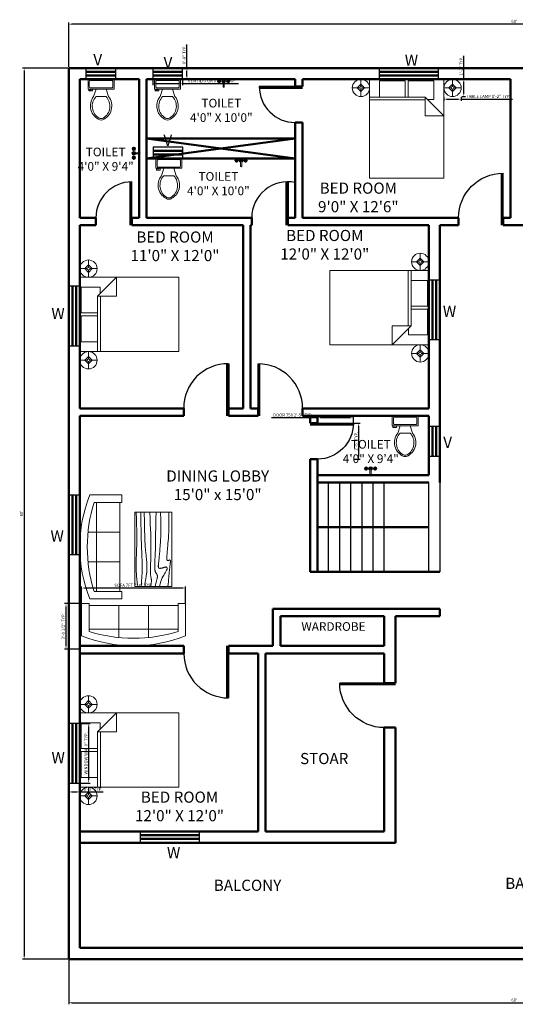
# Model space of a CAD drawing. Units: inches. Extents: x 2663 to 4539, y 2314 to 3111.
# Tile 3 of 4: x 3742 to 4143, y 2316 to 3111. Entities that reach past the tile are written whole.
import ezdxf

# ---------------------------------------------------------------- set-up
doc = ezdxf.new("R2010")
doc.units = ezdxf.units.IN
for name, color, linetype, lineweight in [('A-ANNO-DIMS', 2, 'Continuous', 18), ('A-ANNO-TEXT', 7, 'Continuous', 18), ('A-AREA-IDEN', 3, 'Continuous', 25), ('A-DOOR', 4, 'Continuous', 25), ('A-FLOR-FIXT', 8, 'Continuous', 18), ('A-FLOR-STRS', 2, 'Continuous', 25), ('A-FURN', 8, 'Continuous', 18), ('A-GLAZ', 3, 'Continuous', 25), ('A-WALL', 7, 'Continuous', 50)]:
    doc.layers.add(name, color=color, linetype=linetype, lineweight=lineweight)
doc.styles.get("Standard").update_dxf_attribs({"font": 'arial.ttf'})
doc.dimstyles.new('ISO-25', dxfattribs={"dimtxt": 2.5, "dimasz": 2.5, "dimexe": 1.25, "dimexo": 0.625, "dimtad": 1, "dimdec": 0, "dimlunit": 3, "dimtxsty": 'Standard', "dimcen": 2.5, "dimadec": 0, "dimazin": 0, "dimtfac": 1, "dimtdec": 0, "dimtmove": 0, "dimatfit": 3, "dimfxl": 1, "dimarcsym": 0})

# ---------------------------------------------------------------- blocks, each defined once
blk = doc.blocks.new('Toilet - top')
for p, q in [((9.5, -6), (9.5, -2)), ((-10, -8.5), (-8, -8.5)), ((-10, -9.5), (-10, -8.5)), ((-7, -9.5), (-10, -9.5)), ((-8, -8.5), (-8, -8)), ((-7, -8), (-7, -9.5)), ((-4, -8), (-6, -14)), ((4, -14), (-4, -14)), ((4, -8), (6, -14))]:
    blk.add_line(p, q)
blk.add_lwpolyline([(10.5, -8), (10.5, 0), (-10.5, 0), (-10.5, -8)], close=True)
for points in [[(-9.5, -2), (-9.5, -6)], [(8.5, -1), (-8.5, -1)], [(-8.5, -7), (8.5, -7)]]:
    blk.add_lwpolyline(points)
for centre, radius, start, end in [((-8.62, -1.88), 0.884, 81.8699, 188.1301), ((-8.62, -6.12), 0.884, 171.8699, 278.1301), ((8.62, -1.88), 0.884, 351.8699, 98.1301), ((8.62, -6.12), 0.884, 261.8699, 8.1301), ((3.52, -21.58), 12.17, 141.46911, 247.97143), ((4.2, -21.82), 11.33, 136.36773, 238.94682), ((-3.52, -21.58), 12.17, 292.02843, 38.53071), ((-4.2, -21.82), 11.33, 301.05301, 43.63209), ((0, -27.88), 4, 245.73182, 294.26817), ((0, -29), 4, 254.86053, 285.13947)]:
    blk.add_arc(centre, radius, start, end)
blk = doc.blocks.new('Faucet - Bathroom top')
for p, q in [((-4.107, 0.125), (-4.375, 0.125)), ((-3.75, 0.4788), (-3.75, 0.75)), ((-3.5, 0.482), (-3.5, 0.75)), ((-3.1461, 0.125), (-2.875, 0.125)), ((3.143, 0.125), (2.875, 0.125)), ((3.5, 0.4788), (3.5, 0.75)), ((3.75, 0.482), (3.75, 0.75)), ((4.1039, 0.125), (4.375, 0.125)), ((-4.1039, -0.125), (-4.375, -0.125)), ((-3.75, -0.4821), (-3.75, -0.75)), ((-3.5, -0.4789), (-3.5, -0.75)), ((-3.143, -0.125), (-2.875, -0.125)), ((-0.5, -0.8639), (-0.5, -4.5)), ((0.5, -4.5), (0.5, -0.8631)), ((3.1461, -0.125), (2.875, -0.125)), ((3.5, -0.4821), (3.5, -0.75)), ((3.75, -0.4789), (3.75, -0.75)), ((4.107, -0.125), (4.375, -0.125))]:
    blk.add_line(p, q)
for centre, radius in [((-3.625, 0), 1.375), ((-4.625, 0), 0.2795), ((-3.625, 0), 0.5), ((-3.625, 1), 0.2795), ((-2.625, 0), 0.2795), ((0, 0), 0.5), ((3.625, 0), 1.375), ((2.625, 0), 0.2795), ((3.625, 0), 0.5), ((3.625, 1), 0.2795), ((4.625, 0), 0.2795), ((-3.625, -1), 0.2795), ((3.625, -1), 0.2795)]:
    blk.add_circle(centre, radius)
for centre, radius, start, end in [((-3.625, 0), 1, 105.2407, 164.2093), ((-3.625, 0), 1, 16.44125, 74.07887), ((0, 0), 1.5, 289.6514, 250.3603), ((0, 0), 1, 300.3431, 239.7554), ((3.625, 0), 1, 106.12, 164.0884), ((3.625, 0), 1, 16.23422, 73.90469), ((-3.625, 0), 1, 196.2342, 253.9047), ((-3.625, 0), 1, 286.12, 344.0884), ((0, -4.5), 0.5, 180, 0), ((3.625, 0), 1, 196.4413, 254.0789), ((3.625, 0), 1, 285.2407, 344.2093)]:
    blk.add_arc(centre, radius, start, end)
blk = doc.blocks.new('Bed - Queen')
for p, q in [((0, -80.00003), (0, 0)), ((0, 0), (59.99999, 0)), ((59.99999, 0), (59.99999, -80.00003)), ((7.99999, -1.2), (28.79998, -1.2)), ((7.99999, -14.4), (7.99999, -1.2)), ((28.79998, -1.2), (28.79998, -14.4)), ((31.19999, -1.2), (51.99999, -1.2)), ((31.19999, -14.4), (31.19999, -1.2)), ((51.99999, -1.2), (51.99999, -16.4)), ((0, -14.4), (44.8, -14.4)), ((59.99999, -29.6), (44.8, -14.4)), ((44.8, -14.4), (44.8, -29.6)), ((44.8, -16.8), (0, -16.8)), ((51.99999, -16.4), (46.79936, -16.4)), ((44.8, -29.6), (59.99999, -29.6)), ((59.99999, -80.00003), (0, -80.00003))]:
    blk.add_line(p, q)
blk = doc.blocks.new('Lamp - Table')
for p, q in [((-1, 0), (-7, 0)), ((0, 3), (-3, 0)), ((-3, 0), (0, -3)), ((0, 7), (0, 1)), ((3, 0), (0, 3)), ((0, -3), (3, 0)), ((1, 0), (7, 0)), ((0, -1), (0, -7))]:
    blk.add_line(p, q)
for radius in [7, 1]:
    blk.add_circle((0, 0), radius)
blk = doc.blocks.new('Sofa - Roundback 7 ft.')
for p, q in [((-12.00002, -32.4421), (-12.00003, -6.5971)), ((11.99997, -32.4421), (11.99998, -6.5971)), ((-36.000027, -34), (-36.000027, -11.4696)), ((-35.999844, -13.3819), (35.9998, -13.3819)), ((35.99998, -34), (35.99998, -11.4696)), ((-36.000027, -32.4421), (35.99998, -32.4421))]:
    blk.add_line(p, q)
for points in [[(-36.000027, -34), (-42.000027, -34), (-42.000027, -8)], [(41.99998, -8), (41.99998, -34), (35.99998, -34)]]:
    blk.add_lwpolyline(points)
for centre, radius, start, end in [((0, -114.25), 114.25, 68.43141, 111.5686), ((-0.00001, -127.1968), 121.1968, 72.72033, 107.2797)]:
    blk.add_arc(centre, radius, start, end)
blk = doc.blocks.new('Table - Rectangular Woodgrain 60 x 30 in.')
for p, q in [((0, 0), (0, -30)), ((60, 0), (0, 0)), ((60, -30), (60, 0)), ((0, -30), (60, -30))]:
    blk.add_line(p, q)
for points in [[(0, -2.4), (4.8155, -2.418), (9.0302, -2.4688), (12.709, -2.5477), (15.9167, -2.65), (18.7181, -2.7711), (21.1781, -2.9063), (23.3616, -3.0508), (25.3333, -3.2), (27.1477, -3.3495), (28.8172, -3.4958), (30.3437, -3.636), (31.7291, -3.7667), (32.9756, -3.8849), (34.0849, -3.9875), (35.059, -4.0714), (35.9, -4.1334), (36.6114, -4.1711), (37.2041, -4.1854), (37.6906, -4.1779), (38.0833, -4.15), (38.3948, -4.1034), (38.6375, -4.0396), (38.8239, -3.9602), (38.9666, -3.8667), (39.0764, -3.7608), (39.1573, -3.6448), (39.2116, -3.521), (39.2416, -3.3917), (39.2498, -3.2593), (39.2385, -3.1261), (39.21, -2.9944), (39.1666, -2.8667), (39.111, -2.7447), (39.0468, -2.6281), (38.978, -2.5163), (38.9083, -2.4083), (38.8418, -2.3035), (38.7823, -2.201), (38.7337, -2.1001), (38.7, -2), (38.6844, -1.9003), (38.6875, -1.8021), (38.7094, -1.707), (38.75, -1.6167), (38.8094, -1.5326), (38.8875, -1.4563), (38.9844, -1.3893), (39.1, -1.3333), (39.2351, -1.2896), (39.3937, -1.2583), (39.5804, -1.2396), (39.8, -1.2333), (40.057, -1.2396), (40.3562, -1.2583), (40.7023, -1.2896), (41.1, -1.3333), (41.5547, -1.3895), (42.0755, -1.4573), (42.6721, -1.5361), (43.3542, -1.625), (44.1316, -1.7233), (45.014, -1.8302), (46.0114, -1.9449), (47.1333, -2.0667), (48.3862, -2.1947), (49.7625, -2.3281), (51.2513, -2.4663), (52.8416, -2.6083), (54.5226, -2.7535), (56.2833, -2.9011), (58.1127, -3.0501), (60, -3.2)], [(0, -9.2), (6.5759, -9.0858), (11.9385, -9.0365), (16.2527, -9.0418), (19.6833, -9.0917), (22.3952, -9.1759), (24.5531, -9.2844), (26.322, -9.4069), (27.8666, -9.5333), (29.3241, -9.6553), (30.7203, -9.7719), (32.0532, -9.8837), (33.3208, -9.9917), (34.5213, -10.0965), (35.6526, -10.199), (36.7128, -10.2999), (37.7, -10.4), (38.6129, -10.4996), (39.4531, -10.5969), (40.223, -10.6895), (40.925, -10.775), (41.5613, -10.8512), (42.1344, -10.9156), (42.6465, -10.966), (43.1, -11), (43.4976, -11.0158), (43.8437, -11.0136), (44.143, -10.9942), (44.4, -10.9583), (44.6195, -10.9069), (44.8062, -10.8406), (44.9648, -10.7603), (45.1, -10.6667), (45.2155, -10.5598), (45.3114, -10.4365), (45.3871, -10.2929), (45.4416, -10.125), (45.4743, -9.929), (45.4844, -9.7011), (45.4709, -9.4371), (45.4333, -9.1333), (45.3716, -8.7883), (45.2896, -8.4104), (45.1919, -8.0107), (45.0833, -7.6), (44.9685, -7.1893), (44.8521, -6.7896), (44.7388, -6.4117), (44.6333, -6.0667), (44.54, -5.7628), (44.4614, -5.4979), (44.4001, -5.2675), (44.3583, -5.0667), (44.3384, -4.8909), (44.3427, -4.7354), (44.3736, -4.5956), (44.4333, -4.4667), (44.5236, -4.3453), (44.6427, -4.2333), (44.7884, -4.1339), (44.9583, -4.05), (45.1501, -3.9849), (45.3614, -3.9417), (45.59, -3.9234), (45.8333, -3.9333), (46.0915, -3.9749), (46.3734, -4.0531), (46.6906, -4.1736), (47.0542, -4.3417), (47.4756, -4.5629), (47.9661, -4.8427), (48.5372, -5.1866), (49.2, -5.6), (49.9676, -6.0844), (50.8594, -6.625), (51.8965, -7.2031), (53.1, -7.8), (54.491, -8.3969), (56.0906, -8.975), (57.9199, -9.5156), (60, -10)], [(0, -12.8), (5.1847, -12.9322), (9.6213, -13.0323), (13.3963, -13.1059), (16.5958, -13.1583), (19.3063, -13.1952), (21.614, -13.2219), (23.6054, -13.2439), (25.3666, -13.2667), (26.9728, -13.2947), (28.4531, -13.3281), (29.8256, -13.3663), (31.1083, -13.4083), (32.3191, -13.4535), (33.476, -13.501), (34.597, -13.5501), (35.7, -13.6), (36.7984, -13.6497), (37.8875, -13.6979), (38.9578, -13.743), (40, -13.7833), (41.0047, -13.8174), (41.9625, -13.8438), (42.864, -13.8607), (43.7, -13.8667), (44.4631, -13.8604), (45.1552, -13.8417), (45.7801, -13.8104), (46.3416, -13.7667), (46.8439, -13.7104), (47.2906, -13.6417), (47.6858, -13.5604), (48.0333, -13.4667), (48.3375, -13.3608), (48.6042, -13.2448), (48.8396, -13.121), (49.05, -12.9917), (49.2417, -12.8593), (49.4208, -12.7261), (49.5937, -12.5944), (49.7667, -12.4667), (49.9452, -12.3451), (50.1323, -12.2313), (50.3303, -12.1268), (50.5416, -12.0333), (50.7686, -11.9524), (51.0135, -11.8854), (51.2788, -11.8341), (51.5666, -11.8), (51.8785, -11.7843), (52.2116, -11.7865), (52.562, -11.8059), (52.926, -11.8417), (53.2998, -11.8931), (53.6795, -11.9594), (54.0614, -12.0397), (54.4416, -12.1333), (54.8223, -12.2401), (55.2293, -12.3625), (55.6942, -12.5037), (56.2489, -12.6667), (56.9251, -12.8547), (57.7545, -13.0708), (58.7689, -13.3182), (60, -13.6)], [(0, -18), (5.124, -17.7273), (9.6609, -17.5057), (13.6705, -17.3303), (17.2125, -17.1958), (20.3467, -17.0973), (23.1328, -17.0297), (25.6307, -16.9878), (27.9, -16.9667), (29.9928, -16.9617), (31.9302, -16.9703), (33.7254, -16.9907), (35.3917, -17.0208), (36.9423, -17.0588), (38.3906, -17.1026), (39.7499, -17.1503), (41.0333, -17.2), (42.2519, -17.2496), (43.4073, -17.2969), (44.4986, -17.3395), (45.525, -17.375), (46.4858, -17.4012), (47.3802, -17.4156), (48.2074, -17.416), (48.9667, -17.4), (49.6583, -17.3662), (50.2872, -17.3167), (50.8595, -17.2547), (51.3812, -17.1833), (51.8584, -17.1057), (52.2971, -17.025), (52.7034, -16.9443), (53.0833, -16.8667), (53.443, -16.7951), (53.789, -16.7313), (54.128, -16.6768), (54.4666, -16.6334), (54.8115, -16.6024), (55.1693, -16.5854), (55.5465, -16.5841), (55.95, -16.6), (56.3828, -16.6337), (56.8346, -16.6823), (57.2915, -16.7418), (57.7396, -16.8084), (58.165, -16.878), (58.5539, -16.9469), (58.8924, -17.0111), (59.1666, -17.0667), (59.3679, -17.1107), (59.5078, -17.1438), (59.6032, -17.1675), (59.6708, -17.1833), (59.7275, -17.193), (59.7901, -17.1979), (59.8753, -17.1998), (60, -17.2)], [(0, -22.4), (8.0098, -22.2501), (14.4094, -22.1011), (19.4168, -21.9535), (23.25, -21.8083), (26.1269, -21.6663), (28.2656, -21.5281), (29.884, -21.3947), (31.2, -21.2667), (32.3967, -21.1448), (33.5172, -21.0292), (34.5697, -20.9198), (35.5625, -20.8167), (36.5037, -20.7198), (37.4015, -20.6292), (38.2642, -20.5448), (39.1, -20.4667), (39.9164, -20.3951), (40.7187, -20.3313), (41.5117, -20.2768), (42.3, -20.2333), (43.0883, -20.2024), (43.8812, -20.1854), (44.6836, -20.1841), (45.5, -20.2), (46.3328, -20.234), (47.1747, -20.2844), (48.0163, -20.3488), (48.8479, -20.425), (49.66, -20.5106), (50.4429, -20.6031), (51.1872, -20.7004), (51.8833, -20.8), (52.5246, -20.8999), (53.1166, -20.9995), (53.6681, -21.0983), (54.1875, -21.1958), (54.6834, -21.2919), (55.1646, -21.3859), (55.6394, -21.4777), (56.1167, -21.5667), (56.6028, -21.6515), (57.0961, -21.7266), (57.5929, -21.7852), (58.0896, -21.8208), (58.5823, -21.8268), (59.0674, -21.7964), (59.5412, -21.723), (60, -21.6)], [(0, -25.2), (8.6355, -25.0504), (15.7026, -24.9031), (21.4049, -24.7606), (25.9458, -24.625), (29.529, -24.4988), (32.3578, -24.3844), (34.6359, -24.284), (36.5667, -24.2), (38.3213, -24.1341), (39.9417, -24.0854), (41.437, -24.0523), (42.8167, -24.0333), (44.0901, -24.0268), (45.2667, -24.0313), (46.3557, -24.0451), (47.3667, -24.0667), (48.309, -24.0947), (49.1928, -24.1287), (50.0284, -24.168), (50.826, -24.2125), (51.5959, -24.2617), (52.3483, -24.3151), (53.0935, -24.3725), (53.8417, -24.4334), (54.6009, -24.497), (55.3699, -24.561), (56.1454, -24.6226), (56.9239, -24.6792), (57.7021, -24.7279), (58.4764, -24.7662), (59.2435, -24.7911), (60, -24.8)], [(0, -28.8), (5.6867, -28.6681), (10.45, -28.5698), (14.407, -28.5012), (17.675, -28.4584), (20.3711, -28.4374), (22.6125, -28.4344), (24.5164, -28.4455), (26.2, -28.4667), (27.762, -28.4947), (29.2276, -28.5281), (30.6033, -28.5663), (31.8958, -28.6084), (33.1118, -28.6535), (34.2578, -28.7011), (35.3405, -28.7501), (36.3666, -28.8), (37.3443, -28.8497), (38.288, -28.8974), (39.2137, -28.9412), (40.1375, -28.9792), (41.0753, -29.0093), (42.0432, -29.0297), (43.0572, -29.0384), (44.1333, -29.0333), (45.2936, -29.0114), (46.5843, -28.9641), (48.0579, -28.8816), (49.7666, -28.7542), (51.7629, -28.5721), (54.0989, -28.3255), (56.8272, -28.0048), (60, -27.6)]]:
    blk.add_lwpolyline(points)
blk = doc.blocks.new('*D14')
at = {"layer": 'A-ANNO-DIMS', "color": 0, "lineweight": -2, "transparency": 16777216}
for p, q in [((3781.84, 3072.75), (3781.84, 3108.85)), ((4499.34, 3107.6), (3784.34, 3107.6)), ((4501.84, 3072.75), (4501.84, 3108.85))]:
    blk.add_line(p, q, dxfattribs=at)
at = {"layer": 'A-ANNO-DIMS', "color": 0, "transparency": 16777216}
for points in [[(3784.34, 3108.02), (3784.34, 3107.19), (3781.84, 3107.6)], [(4499.34, 3108.02), (4499.34, 3107.19), (4501.84, 3107.6)]]:
    blk.add_solid(points, dxfattribs=at)
at = {"layer": 'Defpoints', "color": 0, "transparency": 16777216}
for p in [(3781.84, 3107.6), (3781.84, 3072.12), (4501.84, 3072.12)]:
    blk.add_point(p, dxfattribs=at)
at = {"layer": 'A-ANNO-DIMS', "color": 0, "transparency": 16777216, "insert": (4141.84, 3109.51), "char_height": 2.5, "attachment_point": 5}
blk.add_mtext("60'", dxfattribs=at)
blk = doc.blocks.new('*D16')
at = {"layer": 'A-ANNO-DIMS', "color": 0, "lineweight": -2, "transparency": 16777216}
for p, q in [((3781.21, 3072.12), (3744.61, 3072.12)), ((3745.86, 3069.62), (3745.86, 2354.62)), ((3781.21, 2352.12), (3744.61, 2352.12))]:
    blk.add_line(p, q, dxfattribs=at)
at = {"layer": 'A-ANNO-DIMS', "color": 0, "transparency": 16777216}
for points in [[(3745.45, 3069.62), (3746.28, 3069.62), (3745.86, 3072.12)], [(3745.45, 2354.62), (3746.28, 2354.62), (3745.86, 2352.12)]]:
    blk.add_solid(points, dxfattribs=at)
at = {"layer": 'Defpoints', "color": 0, "transparency": 16777216}
for p in [(3781.84, 3072.12), (3745.86, 2352.12), (3781.84, 2352.12)]:
    blk.add_point(p, dxfattribs=at)
at = {"layer": 'A-ANNO-DIMS', "color": 0, "transparency": 16777216, "insert": (3743.96, 2712.12), "char_height": 2.5, "attachment_point": 5, "rotation": 90}
blk.add_mtext("60'", dxfattribs=at)
blk = doc.blocks.new('*D17')
at = {"layer": 'A-ANNO-DIMS', "color": 0, "lineweight": -2, "transparency": 16777216}
for p, q in [((3781.84, 2352.78), (3781.84, 2315.51)), ((4501.84, 2351.5), (4501.84, 2315.51)), ((3784.34, 2316.76), (4499.34, 2316.76))]:
    blk.add_line(p, q, dxfattribs=at)
at = {"layer": 'A-ANNO-DIMS', "color": 0, "transparency": 16777216}
for points in [[(3784.34, 2317.18), (3784.34, 2316.35), (3781.84, 2316.76)], [(4499.34, 2317.18), (4499.34, 2316.35), (4501.84, 2316.76)]]:
    blk.add_solid(points, dxfattribs=at)
at = {"layer": 'Defpoints', "color": 0, "transparency": 16777216}
for p in [(3781.84, 2353.4), (4501.84, 2352.12), (4501.84, 2316.76)]:
    blk.add_point(p, dxfattribs=at)
at = {"layer": 'A-ANNO-DIMS', "color": 0, "transparency": 16777216, "insert": (4141.84, 2318.67), "char_height": 2.5, "attachment_point": 5}
blk.add_mtext("60'", dxfattribs=at)
blk = doc.blocks.new('WIN-1200')
for p, q in [((0, 48), (0, 0)), ((9, 48), (0, 48)), ((0, 48), (0, 48)), ((9, 0), (9, 48)), ((0, 0), (9, 0))]:
    blk.add_line(p, q)
blk = doc.blocks.new('VENT-600')
for p, q in [((24, 9), (0, 9)), ((0, 9), (0, 0)), ((24, 0), (24, 9)), ((0, 0), (24, 0))]:
    blk.add_line(p, q)
blk = doc.blocks.new('DOOR-750')
blk.add_line((2901.63, 3055.91), (2872.63, 3055.91))
blk.add_arc((2901.63, 3055.91), 29, 180, 270)
blk = doc.blocks.new('DOOR-900')
blk.add_line((3071.63, 2949.91), (3071.63, 2985.91))
blk.add_arc((3071.63, 2949.91), 36, 0, 90)
blk = doc.blocks.new('*D24')
at = {"layer": 'A-ANNO-DIMS', "color": 0, "lineweight": -2, "transparency": 16777216}
for p, q in [((4084.96, 3048.5), (4084.96, 3045.77)), ((4098.96, 3048.5), (4098.96, 3045.77)), ((4087.46, 3047.02), (4096.46, 3047.02)), ((4098.96, 3047.02), (4140.53, 3047.02))]:
    blk.add_line(p, q, dxfattribs=at)
at = {"layer": 'A-ANNO-DIMS', "color": 0, "transparency": 16777216}
for points in [[(4087.46, 3047.44), (4087.46, 3046.61), (4084.96, 3047.02)], [(4096.46, 3047.44), (4096.46, 3046.61), (4098.96, 3047.02)]]:
    blk.add_solid(points, dxfattribs=at)
at = {"layer": 'Defpoints', "color": 0, "transparency": 16777216}
for p in [(4084.96, 3049.12), (4098.96, 3049.12), (4098.96, 3047.02)]:
    blk.add_point(p, dxfattribs=at)
at = {"layer": 'A-ANNO-DIMS', "color": 0, "transparency": 16777216, "insert": (4120.99, 3048.91), "char_height": 2.5, "attachment_point": 5}
blk.add_mtext('TABLE LAMP 1\'-2" TYP.', dxfattribs=at)
blk = doc.blocks.new('*D25')
at = {"layer": 'A-ANNO-DIMS', "color": 0, "lineweight": -2, "transparency": 16777216}
for p, q in [((4101.06, 3063.12), (4101.06, 3081.88)), ((4099.58, 3063.12), (4102.31, 3063.12)), ((4101.06, 3051.62), (4101.06, 3060.62)), ((4099.58, 3049.12), (4102.31, 3049.12))]:
    blk.add_line(p, q, dxfattribs=at)
at = {"layer": 'A-ANNO-DIMS', "color": 0, "transparency": 16777216}
for points in [[(4100.64, 3060.62), (4101.48, 3060.62), (4101.06, 3063.12)], [(4100.64, 3051.62), (4101.48, 3051.62), (4101.06, 3049.12)]]:
    blk.add_solid(points, dxfattribs=at)
at = {"layer": 'Defpoints', "color": 0, "transparency": 16777216}
for p in [(4098.96, 3063.12), (4101.06, 3063.12), (4098.96, 3049.12)]:
    blk.add_point(p, dxfattribs=at)
at = {"layer": 'A-ANNO-DIMS', "color": 0, "transparency": 16777216, "insert": (4099.18, 3073.75), "char_height": 2.5, "attachment_point": 5, "rotation": 90}
blk.add_mtext('1\'-2" TYP.', dxfattribs=at)
blk = doc.blocks.new('*D26')
at = {"layer": 'A-ANNO-DIMS', "color": 0, "lineweight": -2, "transparency": 16777216}
for p, q in [((3791.46, 2542.34), (3799.29, 2542.34)), ((3798.04, 2496.84), (3798.04, 2539.84)), ((3791.46, 2494.34), (3799.29, 2494.34))]:
    blk.add_line(p, q, dxfattribs=at)
at = {"layer": 'A-ANNO-DIMS', "color": 0, "transparency": 16777216}
for points in [[(3797.62, 2539.84), (3798.46, 2539.84), (3798.04, 2542.34)], [(3797.62, 2496.84), (3798.46, 2496.84), (3798.04, 2494.34)]]:
    blk.add_solid(points, dxfattribs=at)
at = {"layer": 'Defpoints', "color": 0, "transparency": 16777216}
for p in [(3790.84, 2542.34), (3798.04, 2542.34), (3790.84, 2494.34)]:
    blk.add_point(p, dxfattribs=at)
at = {"layer": 'A-ANNO-DIMS', "color": 0, "transparency": 16777216, "insert": (3796.12, 2518.34), "char_height": 2.5, "attachment_point": 5, "rotation": 90}
blk.add_mtext('WINDOW W 4\'-0" TYP.', dxfattribs=at)
blk = doc.blocks.new('*D27')
at = {"layer": 'A-ANNO-DIMS', "color": 0, "lineweight": -2, "transparency": 16777216}
for p, q in [((3781.84, 2493.72), (3781.84, 2485.89)), ((3790.84, 2493.72), (3790.84, 2485.89)), ((3784.34, 2487.14), (3788.34, 2487.14)), ((3790.84, 2487.14), (3809.83, 2487.14))]:
    blk.add_line(p, q, dxfattribs=at)
at = {"layer": 'A-ANNO-DIMS', "color": 0, "transparency": 16777216}
for points in [[(3784.34, 2487.56), (3784.34, 2486.73), (3781.84, 2487.14)], [(3788.34, 2487.56), (3788.34, 2486.73), (3790.84, 2487.14)]]:
    blk.add_solid(points, dxfattribs=at)
at = {"layer": 'Defpoints', "color": 0, "transparency": 16777216}
for p in [(3781.84, 2494.34), (3790.84, 2494.34), (3790.84, 2487.14)]:
    blk.add_point(p, dxfattribs=at)
at = {"layer": 'A-ANNO-DIMS', "color": 0, "transparency": 16777216, "insert": (3801.58, 2489.05), "char_height": 2.5, "attachment_point": 5}
blk.add_mtext('0\'-9" TYP.', dxfattribs=at)
blk = doc.blocks.new('*D30')
at = {"layer": 'A-ANNO-DIMS', "color": 0, "lineweight": -2, "transparency": 16777216}
for p, q in [((3849.76, 3062.5), (3849.76, 3058.27)), ((3852.26, 3059.52), (3871.26, 3059.52)), ((3873.76, 3062.5), (3873.76, 3058.27)), ((3873.76, 3059.52), (3919.08, 3059.52))]:
    blk.add_line(p, q, dxfattribs=at)
at = {"layer": 'A-ANNO-DIMS', "color": 0, "transparency": 16777216}
for points in [[(3852.26, 3059.94), (3852.26, 3059.11), (3849.76, 3059.52)], [(3871.26, 3059.94), (3871.26, 3059.11), (3873.76, 3059.52)]]:
    blk.add_solid(points, dxfattribs=at)
at = {"layer": 'Defpoints', "color": 0, "transparency": 16777216}
for p in [(3849.76, 3063.12), (3873.76, 3063.12), (3873.76, 3059.52)]:
    blk.add_point(p, dxfattribs=at)
at = {"layer": 'A-ANNO-DIMS', "color": 0, "transparency": 16777216, "insert": (3897.67, 3061.44), "char_height": 2.5, "attachment_point": 5}
blk.add_mtext('VENTILATOR V 2\'-0" TYP.', dxfattribs=at)
blk = doc.blocks.new('*D31')
at = {"layer": 'A-ANNO-DIMS', "color": 0, "lineweight": -2, "transparency": 16777216}
for p, q in [((3877.36, 3072.12), (3877.36, 3091.11)), ((3874.39, 3072.12), (3878.61, 3072.12)), ((3877.36, 3065.62), (3877.36, 3069.62)), ((3874.39, 3063.12), (3878.61, 3063.12))]:
    blk.add_line(p, q, dxfattribs=at)
at = {"layer": 'A-ANNO-DIMS', "color": 0, "transparency": 16777216}
for points in [[(3876.94, 3069.62), (3877.78, 3069.62), (3877.36, 3072.12)], [(3876.94, 3065.62), (3877.78, 3065.62), (3877.36, 3063.12)]]:
    blk.add_solid(points, dxfattribs=at)
at = {"layer": 'Defpoints', "color": 0, "transparency": 16777216}
for p in [(3873.76, 3072.12), (3877.36, 3072.12), (3873.76, 3063.12)]:
    blk.add_point(p, dxfattribs=at)
at = {"layer": 'A-ANNO-DIMS', "color": 0, "transparency": 16777216, "insert": (3875.46, 3082.87), "char_height": 2.5, "attachment_point": 5, "rotation": 90}
blk.add_mtext('0\'-9" TYP.', dxfattribs=at)
blk = doc.blocks.new('*D38')
at = {"layer": 'A-ANNO-DIMS', "color": 0, "lineweight": -2, "transparency": 16777216}
for p, q in [((3982.84, 2789.47), (3945.73, 2789.47)), ((3982.84, 2785.75), (3982.84, 2790.72)), ((4009.34, 2789.47), (3985.34, 2789.47)), ((4011.84, 2785.75), (4011.84, 2790.72))]:
    blk.add_line(p, q, dxfattribs=at)
at = {"layer": 'A-ANNO-DIMS', "color": 0, "transparency": 16777216}
for points in [[(3985.34, 2789.89), (3985.34, 2789.06), (3982.84, 2789.47)], [(4009.34, 2789.89), (4009.34, 2789.06), (4011.84, 2789.47)]]:
    blk.add_solid(points, dxfattribs=at)
at = {"layer": 'Defpoints', "color": 0, "transparency": 16777216}
for p in [(3982.84, 2789.47), (3982.84, 2785.12), (4011.84, 2785.12)]:
    blk.add_point(p, dxfattribs=at)
at = {"layer": 'A-ANNO-DIMS', "color": 0, "transparency": 16777216, "insert": (3963.03, 2791.39), "char_height": 2.5, "attachment_point": 5}
blk.add_mtext('DOOR 750 2\'-5" TYP.', dxfattribs=at)
blk = doc.blocks.new('*D39')
at = {"layer": 'A-ANNO-DIMS', "color": 0, "lineweight": -2, "transparency": 16777216}
for p, q in [((4012.46, 2785.12), (4017.44, 2785.12)), ((4016.19, 2758.62), (4016.19, 2782.62)), ((4012.46, 2756.12), (4017.44, 2756.12))]:
    blk.add_line(p, q, dxfattribs=at)
at = {"layer": 'A-ANNO-DIMS', "color": 0, "transparency": 16777216}
for points in [[(4015.77, 2782.62), (4016.61, 2782.62), (4016.19, 2785.12)], [(4015.77, 2758.62), (4016.61, 2758.62), (4016.19, 2756.12)]]:
    blk.add_solid(points, dxfattribs=at)
at = {"layer": 'Defpoints', "color": 0, "transparency": 16777216}
for p in [(4011.84, 2785.12), (4016.19, 2785.12), (4011.84, 2756.12)]:
    blk.add_point(p, dxfattribs=at)
at = {"layer": 'A-ANNO-DIMS', "color": 0, "transparency": 16777216, "insert": (4014.29, 2770.62), "char_height": 2.5, "attachment_point": 5, "rotation": 90}
blk.add_mtext('2\'-5" TYP.', dxfattribs=at)
blk = doc.blocks.new('*D42')
at = {"layer": 'A-ANNO-DIMS', "color": 0, "lineweight": -2, "transparency": 16777216}
for p, q in [((3792.26, 2639.92), (3792.26, 2653.14)), ((3873.76, 2651.89), (3794.76, 2651.89)), ((3876.26, 2639.92), (3876.26, 2653.14))]:
    blk.add_line(p, q, dxfattribs=at)
at = {"layer": 'A-ANNO-DIMS', "color": 0, "transparency": 16777216}
for points in [[(3794.76, 2652.31), (3794.76, 2651.47), (3792.26, 2651.89)], [(3873.76, 2652.31), (3873.76, 2651.47), (3876.26, 2651.89)]]:
    blk.add_solid(points, dxfattribs=at)
at = {"layer": 'Defpoints', "color": 0, "transparency": 16777216}
for p in [(3792.26, 2651.89), (3792.26, 2639.29), (3876.26, 2639.29)]:
    blk.add_point(p, dxfattribs=at)
at = {"layer": 'A-ANNO-DIMS', "color": 0, "transparency": 16777216, "insert": (3834.26, 2653.81), "char_height": 2.5, "attachment_point": 5}
blk.add_mtext('SOFA 7FT 7\'-0" TYP.', dxfattribs=at)
blk = doc.blocks.new('*D43')
at = {"layer": 'A-ANNO-DIMS', "color": 0, "lineweight": -2, "transparency": 16777216}
for p, q in [((3791.64, 2639.29), (3778.41, 2639.29)), ((3779.66, 2636.79), (3779.66, 2605.12)), ((3791.64, 2602.62), (3778.41, 2602.62))]:
    blk.add_line(p, q, dxfattribs=at)
at = {"layer": 'A-ANNO-DIMS', "color": 0, "transparency": 16777216}
for points in [[(3779.25, 2636.79), (3780.08, 2636.79), (3779.66, 2639.29)], [(3779.25, 2605.12), (3780.08, 2605.12), (3779.66, 2602.62)]]:
    blk.add_solid(points, dxfattribs=at)
at = {"layer": 'Defpoints', "color": 0, "transparency": 16777216}
for p in [(3792.26, 2639.29), (3779.66, 2602.62), (3792.26, 2602.62)]:
    blk.add_point(p, dxfattribs=at)
at = {"layer": 'A-ANNO-DIMS', "color": 0, "transparency": 16777216, "insert": (3777.74, 2620.96), "char_height": 2.5, "attachment_point": 5, "rotation": 90}
blk.add_mtext('3\'-0 1/2" TYP.', dxfattribs=at)

msp = doc.modelspace()

# ---------------------------------------------------------------- linework, layer by layer
at = {"layer": 'A-DOOR'}
for centre, radius, start, end in [((3958.84, 2951.12), 29.14, 78.11722, 180), ((3910.31, 2797.65), 35.48, 89.15319, 180.84681)]:
    msp.add_arc(centre, radius, start, end, dxfattribs=at)
at = {"layer": 'A-FLOR-STRS'}
for p, q in [((3991.84, 2665.12), (3991.84, 2737.12)), ((4000.84, 2665.12), (4000.84, 2737.12)), ((4009.84, 2665.12), (4009.84, 2737.12)), ((4018.84, 2665.12), (4018.84, 2737.12)), ((4027.84, 2665.12), (4027.84, 2737.12)), ((4036.84, 2665.12), (4036.84, 2737.12)), ((4072.84, 2665.12), (4072.84, 2737.12)), ((4081.84, 2737.12), (4081.84, 2665.12))]:
    msp.add_line(p, q, dxfattribs=at)
at = {"layer": 'A-WALL'}
for p, q in [((3781.84, 3072.12), (4501.84, 3072.12)), ((3781.84, 2352.12), (3781.84, 3072.12)), ((3819.8, 3069.12), (3795.8, 3069.12)), ((3795.8, 3066.12), (3819.8, 3066.12)), ((3873.76, 3069.12), (3849.76, 3069.12)), ((3849.76, 3066.12), (3873.76, 3066.12)), ((4080.74, 3069.12), (4032.74, 3069.12)), ((4032.74, 3066.12), (4080.74, 3066.12)), ((3790.84, 3063.12), (3838.84, 3063.12)), ((3790.84, 2951.12), (3790.84, 3063.12)), ((3838.84, 2951.12), (3838.84, 3063.12)), ((3844.84, 2951.12), (3844.84, 3063.12)), ((3844.84, 3063.12), (3964.84, 3063.12)), ((3964.84, 3056.12), (3935.84, 3056.12)), ((3964.84, 3063.12), (3964.84, 3057.12)), ((3964.84, 3057.12), (3964.84, 3063.12)), ((3964.84, 3057.12), (3970.84, 3057.12)), ((3964.84, 3056.12), (3970.84, 3056.12)), ((3970.84, 3063.12), (4138.84, 3063.12)), ((3970.84, 3057.12), (3970.84, 3063.12)), ((4138.84, 2951.12), (4138.84, 3063.12)), ((3964.84, 2951.12), (3964.84, 3028.12)), ((3970.84, 3028.12), (3964.84, 3028.12)), ((3970.84, 2951.12), (3970.84, 3028.12)), ((3844.84, 3015.12), (3964.84, 3015.12)), ((3844.84, 3015.12), (3964.84, 2999.12)), ((3964.84, 3015.12), (3844.84, 2999.12)), ((3964.84, 2999.12), (3964.84, 3015.12)), ((3874.1, 3005.15), (3850.1, 3005.15)), ((3850.1, 3002.15), (3874.1, 3002.15)), ((3844.84, 2999.12), (3964.84, 2999.12)), ((4131.84, 2951.12), (4131.84, 2987.12)), ((3831.84, 2951.12), (3831.84, 2980.12)), ((3957.84, 2951.12), (3957.84, 2980.12)), ((3958.84, 2951.12), (3958.84, 2980.12)), ((3790.84, 2951.12), (3803.84, 2951.12)), ((3790.84, 2945.12), (3803.84, 2945.12)), ((3790.84, 2797.12), (3790.84, 2945.12)), ((3803.84, 2945.12), (3803.84, 2951.12)), ((3831.84, 2951.12), (3831.84, 2945.12)), ((3838.84, 2951.12), (3832.84, 2951.12)), ((3832.84, 2951.12), (3832.84, 2945.12)), ((3832.84, 2951.12), (3838.84, 2951.12)), ((3832.84, 2945.12), (3922.84, 2945.12)), ((3844.84, 2951.12), (3929.7, 2951.12)), ((3922.84, 2797.12), (3922.84, 2945.12)), ((3928.84, 2797.12), (3928.84, 2945.12)), ((3928.84, 2945.12), (3929.7, 2945.12)), ((3929.7, 2945.12), (3929.7, 2951.12)), ((3957.84, 2951.12), (3957.84, 2945.12)), ((3964.84, 2951.12), (3958.84, 2951.12)), ((3958.84, 2951.12), (3958.84, 2945.12)), ((3958.84, 2951.12), (3964.84, 2951.12)), ((3958.84, 2945.12), (4072.84, 2945.12)), ((3970.84, 2951.12), (4096.84, 2951.12)), ((4072.84, 2797.12), (4072.84, 2945.12)), ((4081.84, 2945.12), (4096.84, 2945.12)), ((4081.84, 2797.12), (4081.84, 2945.12)), ((4096.84, 2945.12), (4096.84, 2951.12)), ((4131.84, 2951.12), (4131.84, 2945.12)), ((4138.84, 2951.12), (4132.84, 2951.12)), ((4132.84, 2951.12), (4132.84, 2945.12)), ((4132.84, 2951.12), (4138.84, 2951.12)), ((4132.84, 2945.12), (4150.84, 2945.12)), ((4075.84, 2900.63), (4075.84, 2852.63)), ((4078.84, 2852.63), (4078.84, 2900.63)), ((3784.84, 2895.77), (3784.84, 2847.77)), ((3787.84, 2847.77), (3787.84, 2895.77)), ((3909.84, 2797.12), (3909.84, 2833.12)), ((3910.84, 2797.12), (3910.84, 2833.12)), ((3935.84, 2797.12), (3935.84, 2833.12)), ((3790.84, 2797.12), (3874.84, 2797.12)), ((3874.84, 2791.12), (3874.84, 2797.12)), ((3909.84, 2797.12), (3909.84, 2791.12)), ((3922.84, 2797.12), (3910.84, 2797.12)), ((3910.84, 2797.12), (3910.84, 2791.12)), ((3910.84, 2797.12), (3922.84, 2797.12)), ((3928.84, 2797.12), (3934.84, 2797.12)), ((3928.84, 2797.12), (3934.84, 2797.12)), ((3934.84, 2797.12), (3934.84, 2791.12)), ((3935.84, 2797.12), (3935.84, 2791.12)), ((3970.84, 2791.12), (3970.84, 2797.12)), ((3970.84, 2797.12), (4072.84, 2797.12)), ((4081.84, 2797.12), (4081.84, 2789.25)), ((3790.84, 2791.12), (3874.84, 2791.12)), ((3790.84, 2635.12), (3790.84, 2791.12)), ((3910.84, 2791.12), (3934.84, 2791.12)), ((3970.84, 2791.12), (4072.84, 2791.12)), ((3976.84, 2791.12), (3976.84, 2785.12)), ((3976.84, 2785.12), (3976.84, 2791.12)), ((3976.84, 2785.12), (3976.84, 2791.12)), ((3976.84, 2785.12), (3982.84, 2785.12)), ((3976.84, 2785.12), (3982.84, 2785.12)), ((3982.84, 2785.12), (3982.84, 2791.12)), ((3982.84, 2785.12), (3982.84, 2791.12)), ((4072.84, 2743.12), (4072.84, 2791.12)), ((4081.84, 2746.12), (4081.84, 2791.12)), ((3976.84, 2784.12), (3982.84, 2784.12)), ((3982.84, 2784.12), (4011.84, 2784.12)), ((4075.84, 2782.39), (4075.84, 2758.39)), ((4078.84, 2758.39), (4078.84, 2782.39)), ((3976.84, 2737.12), (3976.84, 2756.12)), ((3976.84, 2665.12), (3976.84, 2756.12)), ((3982.84, 2756.12), (3976.84, 2756.12)), ((3982.84, 2737.12), (3982.84, 2756.12)), ((3982.84, 2665.12), (3982.84, 2756.12)), ((4081.84, 2746.12), (4081.84, 2737.12)), ((3982.84, 2743.12), (4072.84, 2743.12)), ((3982.84, 2737.12), (4072.84, 2737.12)), ((3784.84, 2726.98), (3784.84, 2678.98)), ((3787.84, 2678.98), (3787.84, 2726.98)), ((3982.84, 2701.12), (4072.84, 2701.12)), ((3982.84, 2665.12), (3976.84, 2665.12)), ((3982.84, 2665.12), (4072.84, 2665.12)), ((4072.84, 2665.12), (4081.84, 2665.12)), ((3790.84, 2605.12), (3790.84, 2635.12)), ((3946.84, 2635.12), (4072.84, 2635.12)), ((3946.84, 2629.12), (3946.84, 2635.12)), ((4072.84, 2635.12), (4081.84, 2635.12)), ((4081.84, 2635.12), (4081.84, 2629.12)), ((3790.84, 2361.12), (3790.84, 2629.12)), ((3946.84, 2605.12), (3946.84, 2629.12)), ((3952.84, 2629.12), (4036.84, 2629.12)), ((3952.84, 2605.12), (3952.84, 2629.12)), ((4036.84, 2605.12), (4036.84, 2629.12)), ((4045.84, 2629.12), (4078.84, 2629.12)), ((4045.84, 2575.12), (4045.84, 2629.12)), ((4081.84, 2629.12), (4078.84, 2629.12)), ((3874.84, 2605.12), (3790.84, 2605.12)), ((3874.84, 2605.12), (3874.84, 2599.12)), ((3909.84, 2599.12), (3909.84, 2605.12)), ((3946.84, 2605.12), (3910.84, 2605.12)), ((3910.84, 2599.12), (3910.84, 2605.12)), ((3952.84, 2605.12), (4036.84, 2605.12)), ((3874.84, 2599.12), (3790.84, 2599.12)), ((3909.84, 2599.12), (3909.84, 2563.12)), ((3934.84, 2599.12), (3910.84, 2599.12)), ((3934.84, 2599.12), (3910.84, 2599.12)), ((3934.84, 2599.12), (3910.84, 2599.12)), ((3934.84, 2455.12), (3934.84, 2599.12)), ((3946.84, 2599.12), (3940.84, 2599.12)), ((3940.84, 2455.12), (3940.84, 2599.12)), ((3946.84, 2599.12), (4036.84, 2599.12)), ((4036.84, 2599.12), (4036.84, 2575.12)), ((4036.84, 2575.12), (4036.84, 2599.12)), ((4036.84, 2574.12), (4000.84, 2574.12)), ((4036.84, 2575.12), (4045.84, 2575.12)), ((4036.84, 2574.12), (4045.84, 2574.12)), ((3784.84, 2542.34), (3784.84, 2494.34)), ((3787.84, 2494.34), (3787.84, 2542.34)), ((4036.84, 2455.12), (4036.84, 2539.12)), ((4045.84, 2539.12), (4036.84, 2539.12)), ((4045.84, 2446.12), (4045.84, 2539.12)), ((3934.84, 2455.12), (3790.84, 2455.12)), ((3887.49, 2452.12), (3839.49, 2452.12)), ((3946.84, 2455.12), (3940.84, 2455.12)), ((3946.84, 2455.12), (4036.84, 2455.12)), ((3946.84, 2446.12), (3790.84, 2446.12)), ((3839.49, 2449.12), (3887.49, 2449.12)), ((3946.84, 2446.12), (4042.84, 2446.12)), ((4042.84, 2446.12), (4045.84, 2446.12)), ((4237.84, 2361.12), (3790.84, 2361.12)), ((4501.84, 2352.12), (3781.84, 2352.12))]:
    msp.add_line(p, q, dxfattribs=at)

# ---------------------------------------------------------------- block references
at = {"layer": 'A-DOOR'}
for name, p in [('DOOR-750', (1063.21, 1.21)), ('DOOR-900', (863.21, -152.79))]:
    msp.add_blockref(name, p, dxfattribs=at)
at = {"layer": 'A-DOOR', "extrusion": (0, 0, -1), "zscale": -1}
for name, p in [('DOOR-900', (-7204.47, 1.21)), ('DOOR-750', (-6884.47, -270.79))]:
    msp.add_blockref(name, p, dxfattribs=at)
at = {"layer": 'A-DOOR'}
for name, p, rotation in [('DOOR-750', (776.92, 5852.76), 270), ('DOOR-900', (6982.47, 5549.04), 180)]:
    msp.add_blockref(name, p, dxfattribs=dict(at, rotation=rotation))
at = {"layer": 'A-DOOR', "extrusion": (0, 0, -1), "zscale": -1, "rotation": 270.0000000000021}
msp.add_blockref('DOOR-900', (-6986.75, 5646.76), dxfattribs=at)
at = {"layer": 'A-FLOR-FIXT'}
for name, p in [('Toilet - top', (3808.01, 3063.12)), ('Toilet - top', (3861.72, 3063.12)), ('Faucet - Bathroom top', (3907.04, 3061.63)), ('Toilet - top', (3862.72, 2999.12)), ('Faucet - Bathroom top', (3921.11, 2997.4)), ('Toilet - top', (4053.67, 2791.12)), ('Faucet - Bathroom top', (4025.76, 2748.47))]:
    msp.add_blockref(name, p, dxfattribs=at)
at = {"layer": 'A-FLOR-FIXT', "rotation": 90}
msp.add_blockref('Faucet - Bathroom top', (3834.49, 3003.24), dxfattribs=at)
at = {"layer": 'A-FURN'}
for name, p in [('Lamp - Table', (4017.96, 3056.12)), ('Bed - Queen', (4024.96, 3063.12)), ('Lamp - Table', (4091.96, 3056.12))]:
    msp.add_blockref(name, p, dxfattribs=at)
for name, p, rotation in [('Lamp - Table', (4065.84, 2915.53), 270), ('Lamp - Table', (3797.84, 2910.01), 89.99999999999953), ('Bed - Queen', (4072.84, 2908.53), 270), ('Bed - Queen', (3790.84, 2843.01), 89.99999999999953), ('Lamp - Table', (3797.84, 2836.01), 89.99999999999953), ('Lamp - Table', (4065.84, 2841.53), 270), ('Sofa - Roundback 7 ft.', (3790.84, 2685.11), 89.99999999999999), ('Table - Rectangular Woodgrain 60 x 30 in.', (3865.27, 2713.28), 270), ('Sofa - Roundback 7 ft.', (3834.26, 2605.29), 180), ('Lamp - Table', (3797.84, 2557.93), 89.99999999999953), ('Bed - Queen', (3790.84, 2490.93), 89.99999999999953), ('Lamp - Table', (3797.84, 2483.93), 89.99999999999953)]:
    msp.add_blockref(name, p, dxfattribs=dict(at, rotation=rotation))
at = {"layer": 'A-GLAZ'}
for name, p in [('VENT-600', (3795.8, 3063.12)), ('VENT-600', (3849.76, 3063.12)), ('VENT-600', (3850.1, 2999.15)), ('WIN-1200', (4072.84, 2852.63)), ('WIN-1200', (3781.84, 2847.78)), ('WIN-1200', (3781.84, 2678.98)), ('WIN-1200', (3781.84, 2494.35))]:
    msp.add_blockref(name, p, dxfattribs=at)
for name, p, rotation in [('WIN-1200', (4080.74, 3063.12), 89.99999999999666), ('VENT-600', (4072.84, 2782.39), 269.9999999999988), ('WIN-1200', (3887.49, 2446.12), 89.99999999999721)]:
    msp.add_blockref(name, p, dxfattribs=dict(at, rotation=rotation))

# ---------------------------------------------------------------- texts
at = {"layer": 'A-ANNO-TEXT', "char_height": 9, "attachment_point": 1}
for s, insert in [('\\pxqc;V', (3754.55, 3083.4)), ('\\pxqc;V', (3811.31, 3081.12)), ('\\pxqc;W', (4008.02, 3083.03)), ('\\pxqc;V', (3811.16, 3018.23)), ('\\pxqc;W', (3722.48, 2878.31)), ('\\pxqc;W', (4038.8, 2880.01)), ('\\pxqc;V', (4037.27, 2774.12)), ('\\pxqc;W', (3721.79, 2698.51)), ('\\pxqc;W', (3722.61, 2519.37)), ('\\pxqc;W', (3815.87, 2442.6))]:
    msp.add_mtext_dynamic_manual_height_columns(s, width=101.4958, gutter_width=12.5, heights=[0], dxfattribs=dict(at, insert=insert))
at = {"layer": 'A-AREA-IDEN', "attachment_point": 1}
for s, width, insert, char_height in [('\\pxqc;TOILET^J4\'0" X 10\'0"', 66.2554, (3872.04, 3047.29), 7), ('\\pxqc;TOILET^J4\'0" X 9\'4"', 66.2554, (3778.58, 3007.81), 7), ('\\pxqc;TOILET^J4\'0" X 10\'0"', 66.2554, (3869.65, 2988.04), 7), ('\\pxqc;BED ROOM \\P9\'0" X 12\'6"', 107.0744, (3962.3, 2979.6), 9), ('\\pxqc;BED ROOM \\P11\'0" X 12\'0"', 107.0744, (3814.21, 2940.08), 9), ('\\pxqc;BED ROOM \\P12\'0" X 12\'0"', 107.0744, (3935.22, 2941.33), 9), ('\\pxqc;TOILET^J4\'0" X 9\'4"', 66.2554, (3992.82, 2771.59), 7), ('\\pxqc;DINING LOBBY\\P15\'0" x 15\'0"', 101.6643, (3851.38, 2746.96), 9), ('\\pxqc;WARDROBE', 73.6922, (3958.93, 2624.33), 7), ('\\pxqc;STOAR', 82.7658, (3946.93, 2518.62), 9), ('\\pxqc;BED ROOM \\P12\'0" X 12\'0"', 107.0744, (3817.85, 2487.44), 9), ('\\pxqc;BALCONY', 201.8325, (3825.43, 2416.21), 9), ('\\pxqc;BALCONY', 201.8325, (4060.93, 2417.75), 9)]:
    msp.add_mtext_dynamic_manual_height_columns(s, width=width, gutter_width=12.5, heights=[0], dxfattribs=dict(at, insert=insert, char_height=char_height))

# ---------------------------------------------------------------- dimensions: what is measured, and where the dimension line sits
at = {"layer": 'A-ANNO-DIMS'}
for base, p1, p2, picture, middle in [((3781.84, 3107.6), (4501.84, 3072.12), (3781.84, 3072.12), '*D14', (4141.84, 3109.51)), ((4501.84, 2316.76), (3781.84, 2353.4), (4501.84, 2352.12), '*D17', (4141.84, 2318.67))]:
    dim = msp.add_linear_dim(base=base, p1=p1, p2=p2, dimstyle='ISO-25', override={"dimclrd": 0, "dimclre": 0, "dimclrt": 0}, dxfattribs=at)
    dim.commit()
    dim.dimension.update_dxf_attribs({"geometry": picture, "text_midpoint": middle})
for base, p1, p2, angle, text, picture, middle in [((3877.36, 3072.12), (3873.76, 3063.12), (3873.76, 3072.12), 90, '<> TYP.', '*D31', (3875.46, 3082.87)), ((4101.06, 3063.12), (4098.96, 3049.12), (4098.96, 3063.12), 90, '<> TYP.', '*D25', (4099.18, 3073.75)), ((3982.84, 2789.47), (4011.84, 2785.12), (3982.84, 2785.12), 180, 'DOOR 750 <> TYP.', '*D38', (3963.03, 2791.39)), ((4016.19, 2785.12), (4011.84, 2756.12), (4011.84, 2785.12), 90, '<> TYP.', '*D39', (4014.29, 2770.62)), ((3792.26, 2651.89), (3876.26, 2639.29), (3792.26, 2639.29), 180, 'SOFA 7FT <> TYP.', '*D42', (3834.26, 2653.81)), ((3779.66, 2602.62), (3792.26, 2639.29), (3792.26, 2602.62), 270, '<> TYP.', '*D43', (3777.74, 2620.96)), ((3798.04, 2542.34), (3790.84, 2494.34), (3790.84, 2542.34), 90, 'WINDOW W <> TYP.', '*D26', (3796.12, 2518.34))]:
    dim = msp.add_linear_dim(base=base, p1=p1, p2=p2, angle=angle, text=text, dimstyle='ISO-25', override={"dimdec": 1, "dimrnd": 0, "dimzin": 1, "dimlunit": 4, "dimfrac": 2}, dxfattribs=at)
    dim.commit()
    dim.dimension.update_dxf_attribs({"geometry": picture, "text_midpoint": middle})
dim = msp.add_linear_dim(base=(3745.86, 2352.12), p1=(3781.84, 3072.12), p2=(3781.84, 2352.12), angle=90, dimstyle='ISO-25', override={"dimclrd": 0, "dimclre": 0, "dimclrt": 0}, dxfattribs=at)
dim.commit()
dim.dimension.update_dxf_attribs({"geometry": '*D16', "text_midpoint": (3743.96, 2712.12)})
for base, p1, p2, text, picture, middle in [((3873.76, 3059.52), (3849.76, 3063.12), (3873.76, 3063.12), 'VENTILATOR V <> TYP.', '*D30', (3897.67, 3061.44)), ((4098.96, 3047.02), (4084.96, 3049.12), (4098.96, 3049.12), 'TABLE LAMP <> TYP.', '*D24', (4120.99, 3048.91)), ((3790.84, 2487.14), (3781.84, 2494.34), (3790.84, 2494.34), '<> TYP.', '*D27', (3801.58, 2489.05))]:
    dim = msp.add_linear_dim(base=base, p1=p1, p2=p2, text=text, dimstyle='ISO-25', override={"dimdec": 1, "dimrnd": 0, "dimzin": 1, "dimlunit": 4, "dimfrac": 2}, dxfattribs=at)
    dim.commit()
    dim.dimension.update_dxf_attribs({"geometry": picture, "text_midpoint": middle})

doc.saveas('drawing.dxf')
